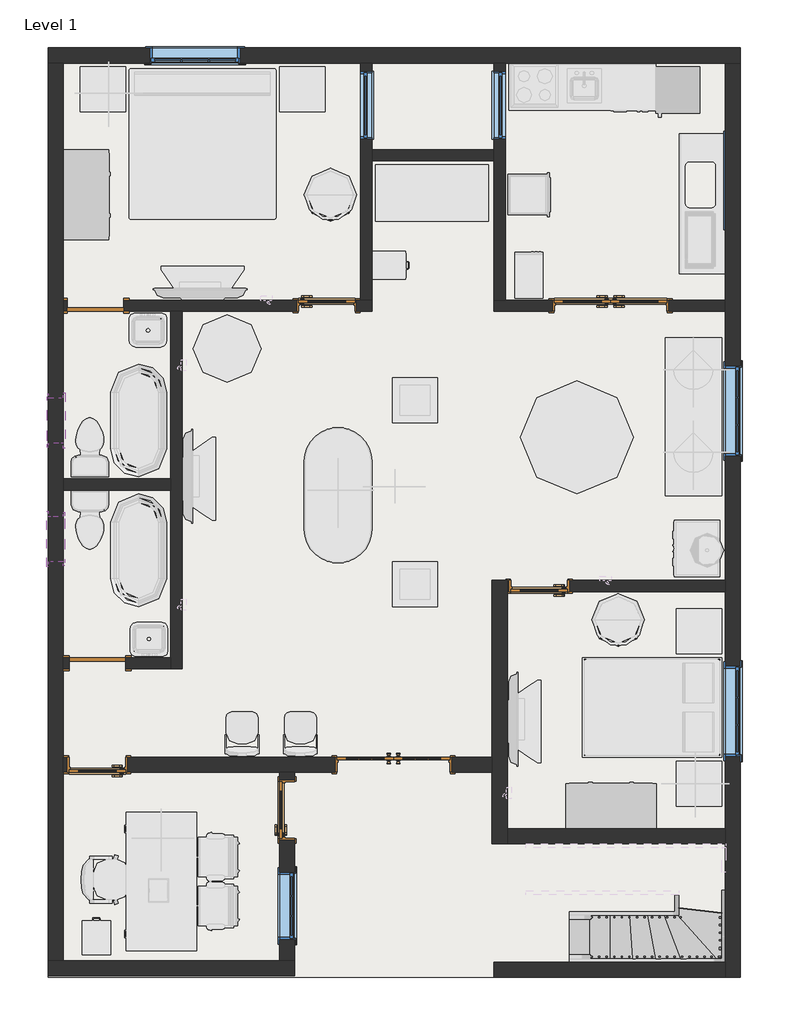
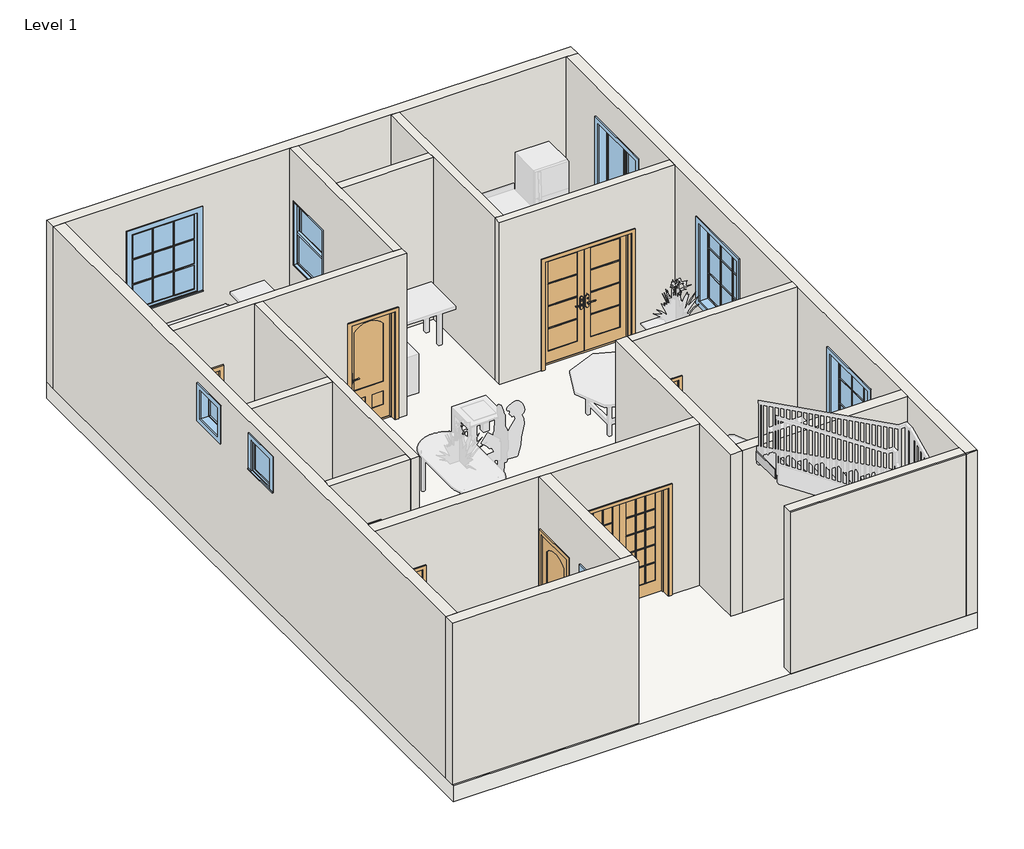
# One storey, part 1 of 3: 18 walls, 9 windows, 8 doors, 1 slab, 1 stair flight.
"""IFC4 building model written with IfcOpenShell, lengths in millimetres."""

from ifc_helpers import new_model, si_unit, frame, origin, origin_with_axes, place, context, project, spatial, polyline, outline, extrude, faceted_brep, transform, mapped, element, save
from components import door_41326d50, door_4b146b56, door_94998e6c, door_9d00318c, door_255cab33, door_059fdd7e, stair_flight_08a12ea7, window_29c06734, window_4f803b43, window_cfa1ffdd, window_0862ab64, window_d6fe7540, window_e41d21a6

model = new_model("IFC4")

# Units and contexts
model_context = context("Model", 3, world=origin())
ifc_project = project(units=[si_unit("LENGTHUNIT", "METRE", prefix="MILLI")], contexts=[model_context])

# Site, building, storey
site = spatial("IfcSite", under=ifc_project)
building = spatial("IfcBuilding", under=site)
storey = spatial("IfcBuildingStorey", under=building, Name="Level 1", Elevation=0.0)

# Doors
placement = place(None, origin())
door_shape = door_41326d50(model_context)
element("IfcDoor", 1, ObjectType="30\" x 80\"", at=placement, inside=storey, context=model_context, shape_type="MappedRepresentation", body=[
    mapped(door_shape, transform((-5998.3041596, 3065.8845092, 0.0), x_axis=(1.0, 0.0, 0.0), y_axis=(0.0, 1.0, 0.0), z_axis=(0.0, 0.0, 1.0))),
])
element("IfcDoor", 2, ObjectType="30\" x 80\"", at=placement, inside=storey, context=model_context, shape_type="MappedRepresentation", body=[
    mapped(door_shape, transform((-3436.0791596, 2459.4595092, 0.0), x_axis=(0.0, -1.0, 0.0), y_axis=(1.0, 0.0, 0.0), z_axis=(0.0, 0.0, 1.0))),
])
door_2_shape = door_4b146b56(model_context)
element("IfcDoor", 3, ObjectType="30\" x 80\"", at=placement, inside=storey, context=model_context, shape_type="MappedRepresentation", body=[
    mapped(door_2_shape, transform((-29.3041596, 5478.8845092, 0.0), x_axis=(1.0, 0.0, 0.0), y_axis=(0.0, 1.0, 0.0), z_axis=(0.0, 0.0, 1.0))),
])
element("IfcDoor", 4, ObjectType="30\" x 80\"", at=placement, inside=storey, context=model_context, shape_type="MappedRepresentation", body=[
    mapped(door_2_shape, transform((-2899.5041596, 9269.8345092, 0.0), x_axis=(-1.0, 0.0, 0.0), y_axis=(0.0, -1.0, 0.0), z_axis=(0.0, 0.0, 1.0))),
])
door_3_shape = door_94998e6c(model_context)
element("IfcDoor", 5, ObjectType="Door-Exterior-Double-Full Glass-Wood_Clad : 60\" x 80\"", at=placement, inside=storey, context=model_context, shape_type="MappedRepresentation", body=[
    mapped(door_3_shape, transform((935.8958404, 9269.8345092, 0.0), x_axis=(1.0, 0.0, 0.0), y_axis=(0.0, 1.0, 0.0), z_axis=(0.0, 0.0, 1.0))),
])
door_4_shape = door_9d00318c(model_context)
element("IfcDoor", 6, ObjectType="Door-Interior-Double-Full Glass-Wood : 60\" x 80\"", at=placement, inside=storey, context=model_context, shape_type="MappedRepresentation", body=[
    mapped(door_4_shape, transform((-1997.8041596, 3072.2345092, 0.0), x_axis=(1.0, 0.0, 0.0), y_axis=(0.0, 1.0, 0.0), z_axis=(0.0, 0.0, 1.0))),
])
door_5_shape = door_255cab33(model_context)
element("IfcDoor", 7, ObjectType="Single-Flush : 30\" x 80\"", at=placement, inside=storey, context=model_context, shape_type="MappedRepresentation", body=[
    mapped(door_5_shape, transform((-5998.3041596, 4440.6595092, 0.0), x_axis=(-1.0, 0.0, 0.0), y_axis=(0.0, -1.0, 0.0), z_axis=(0.0, 0.0, 1.0))),
])
door_6_shape = door_059fdd7e(model_context)
element("IfcDoor", 8, ObjectType="Single-Flush : 30\" x 80\"", at=placement, inside=storey, context=model_context, shape_type="MappedRepresentation", body=[
    mapped(door_6_shape, transform((-6023.7041596, 9266.6595092, 0.0), x_axis=(-1.0, 0.0, 0.0), y_axis=(0.0, -1.0, 0.0), z_axis=(0.0, 0.0, 1.0))),
])

# Slab
element("IfcSlab", 9, ObjectType="Generic - 12\"", at=placement, inside=storey, context=model_context, shape_type="SweptSolid", body=[
    extrude(outline(polyline([(2688.4958404, 12746.4595092), (2688.4958404, 198.8595092), (-6658.7041596, 198.8595092), (-6658.7041596, 12746.4595092), (2688.4958404, 12746.4595092)])), frame((0.0, 0.0, -304.8), z_axis=(0.0, 0.0, 1.0), x_axis=(1.0, 0.0, 0.0)), (0.0, 0.0, 1.0), 304.8),
])

# Stair flight
stair_flight_shape = stair_flight_08a12ea7(model_context)
element("IfcStairFlight", 10, ObjectType="2\" Tread 1\" Nosing 1/4\" Riser", at=placement, inside=storey, context=model_context, shape_type="MappedRepresentation", body=[
    mapped(stair_flight_shape, transform((0.0, 0.0, 0.0), x_axis=(1.0, 0.0, 0.0), y_axis=(0.0, 1.0, 0.0), z_axis=(0.0, 0.0, 1.0))),
])

# Walls
element("IfcWall", 11, ObjectType="Generic - 8\"", at=placement, inside=storey, context=model_context, shape_type="Brep", body=[
    faceted_brep([(-6658.7041596, 12543.2595092, 0.0), (-6455.5041596, 12543.2595092, 0.0), (-2442.3041596, 12543.2595092, 0.0), (-2289.9041596, 12543.2595092, 0.0), (-638.9041596, 12543.2595092, 0.0), (-486.5041596, 12543.2595092, 0.0), (2485.2958404, 12543.2595092, 0.0), (2688.4958404, 12543.2595092, 0.0), (2688.4958404, 12543.2595092, 3048.0), (2485.2958404, 12543.2595092, 3048.0), (-486.5041596, 12543.2595092, 3048.0), (-638.9041596, 12543.2595092, 3048.0), (-2289.9041596, 12543.2595092, 3048.0), (-2442.3041596, 12543.2595092, 3048.0), (-6455.5041596, 12543.2595092, 3048.0), (-6658.7041596, 12543.2595092, 3048.0), (-4067.9041596, 12543.2595092, 2438.4), (-4067.9041596, 12543.2595092, 914.4), (-5287.1041596, 12543.2595092, 914.4), (-5287.1041596, 12543.2595092, 2438.4), (-6658.7041596, 12746.4595092, 0.0), (-6658.7041596, 12746.4595092, 3048.0), (2688.4958404, 12746.4595092, 3048.0), (2688.4958404, 12746.4595092, 0.0), (-4067.9041596, 12746.4595092, 2438.4), (-5287.1041596, 12746.4595092, 2438.4), (-5287.1041596, 12746.4595092, 914.4), (-4067.9041596, 12746.4595092, 914.4)], [[[0, 1, 2, 3, 4, 5, 6, 7, 8, 9, 10, 11, 12, 13, 14, 15], [16, 17, 18, 19]], [[20, 21, 22, 23], [24, 25, 26, 27]], [[7, 6, 5, 4, 3, 2, 1, 0, 20, 23]], [[8, 7, 23, 22]], [[0, 15, 21, 20]], [[15, 14, 13, 12, 11, 10, 9, 8, 22, 21]], [[17, 16, 24, 27]], [[18, 17, 27, 26]], [[19, 18, 26, 25]], [[16, 19, 25, 24]]]),
])
element("IfcWall", 12, ObjectType="Generic - 8\"", at=placement, inside=storey, context=model_context, shape_type="Brep", body=[
    faceted_brep([(2485.2958404, 12543.2595092, 0.0), (2485.2958404, 9342.8595092, 0.0), (2485.2958404, 9190.4595092, 0.0), (2485.2958404, 5558.2595092, 0.0), (2485.2958404, 5405.8595092, 0.0), (2485.2958404, 2205.4595092, 0.0), (2485.2958404, 2002.2595092, 0.0), (2485.2958404, 402.0595092, 0.0), (2485.2958404, 198.8595092, 0.0), (2485.2958404, 198.8595092, 3048.0), (2485.2958404, 224.2595092, 3048.0), (2485.2958404, 402.0595092, 3048.0), (2485.2958404, 2002.2595092, 3048.0), (2485.2958404, 2205.4595092, 3048.0), (2485.2958404, 5405.8595092, 3048.0), (2485.2958404, 5558.2595092, 3048.0), (2485.2958404, 9190.4595092, 3048.0), (2485.2958404, 9342.8595092, 3048.0), (2485.2958404, 12543.2595092, 3048.0), (2485.2958404, 3183.3595092, 2438.4), (2485.2958404, 3183.3595092, 914.4), (2485.2958404, 4402.5595092, 914.4), (2485.2958404, 4402.5595092, 2438.4), (2485.2958404, 7234.6595092, 2438.4), (2485.2958404, 7234.6595092, 914.4), (2485.2958404, 8453.8595092, 914.4), (2485.2958404, 8453.8595092, 2438.4), (2485.2958404, 10346.1595092, 2438.4), (2485.2958404, 10346.1595092, 1219.2), (2485.2958404, 11565.3595092, 1219.2), (2485.2958404, 11565.3595092, 2438.4), (2688.4958404, 12543.2595092, 0.0), (2688.4958404, 12543.2595092, 3048.0), (2688.4958404, 224.2595092, 3048.0), (2688.4958404, 198.8595092, 3048.0), (2688.4958404, 198.8595092, 0.0), (2688.4958404, 3183.3595092, 2438.4), (2688.4958404, 4402.5595092, 2438.4), (2688.4958404, 4402.5595092, 914.4), (2688.4958404, 3183.3595092, 914.4), (2688.4958404, 7234.6595092, 2438.4), (2688.4958404, 8453.8595092, 2438.4), (2688.4958404, 8453.8595092, 914.4), (2688.4958404, 7234.6595092, 914.4), (2688.4958404, 10346.1595092, 2438.4), (2688.4958404, 11565.3595092, 2438.4), (2688.4958404, 11565.3595092, 1219.2), (2688.4958404, 10346.1595092, 1219.2)], [[[0, 1, 2, 3, 4, 5, 6, 7, 8, 9, 10, 11, 12, 13, 14, 15, 16, 17, 18], [19, 20, 21, 22], [23, 24, 25, 26], [27, 28, 29, 30]], [[31, 32, 33, 34, 35], [36, 37, 38, 39], [40, 41, 42, 43], [44, 45, 46, 47]], [[8, 7, 6, 5, 4, 3, 2, 1, 0, 31, 35]], [[0, 18, 32, 31]], [[9, 8, 35, 34]], [[10, 9, 34, 33]], [[18, 17, 16, 15, 14, 13, 12, 11, 10, 33, 32]], [[20, 19, 36, 39]], [[21, 20, 39, 38]], [[22, 21, 38, 37]], [[19, 22, 37, 36]], [[24, 23, 40, 43]], [[25, 24, 43, 42]], [[26, 25, 42, 41]], [[23, 26, 41, 40]], [[28, 27, 44, 47]], [[29, 28, 47, 46]], [[30, 29, 46, 45]], [[27, 30, 45, 44]]]),
])
element("IfcWall", 13, ObjectType="Generic - 8\"", at=placement, inside=storey, context=model_context, shape_type="SweptSolid", body=[
    extrude(outline(polyline([(402.0595092, 3048.0), (402.0595092, 0.0), (198.8595092, 0.0), (198.8595092, 3048.0), (224.2595092, 3048.0), (402.0595092, 3048.0)])), frame((-638.9041596, 0.0, 0.0), z_axis=(1.0, 0.0, 0.0), x_axis=(0.0, 1.0, 0.0)), (0.0, 0.0, 1.0), 3124.2),
])
element("IfcWall", 14, ObjectType="Generic - 8\"", at=placement, inside=storey, context=model_context, shape_type="Brep", body=[
    faceted_brep([(-6455.5041596, 427.4595092, 0.0), (-6455.5041596, 2967.4595092, 0.0), (-6455.5041596, 3170.6595092, 0.0), (-6455.5041596, 4364.4595092, 0.0), (-6455.5041596, 4516.8595092, 0.0), (-6455.5041596, 6777.4595092, 0.0), (-6455.5041596, 6929.8595092, 0.0), (-6455.5041596, 9190.4595092, 0.0), (-6455.5041596, 9342.8595092, 0.0), (-6455.5041596, 12543.2595092, 0.0), (-6455.5041596, 12543.2595092, 3048.0), (-6455.5041596, 9342.8595092, 3048.0), (-6455.5041596, 9190.4595092, 3048.0), (-6455.5041596, 6929.8595092, 3048.0), (-6455.5041596, 6777.4595092, 3048.0), (-6455.5041596, 4516.8595092, 3048.0), (-6455.5041596, 4364.4595092, 3048.0), (-6455.5041596, 3170.6595092, 3048.0), (-6455.5041596, 2967.4595092, 3048.0), (-6455.5041596, 427.4595092, 3048.0), (-6455.5041596, 6421.8595092, 2768.6), (-6455.5041596, 6421.8595092, 2159.0), (-6455.5041596, 5812.2595092, 2159.0), (-6455.5041596, 5812.2595092, 2768.6), (-6455.5041596, 7412.4595092, 2768.6), (-6455.5041596, 8022.0595092, 2768.6), (-6455.5041596, 8022.0595092, 2159.0), (-6455.5041596, 7412.4595092, 2159.0), (-6658.7041596, 427.4595092, 0.0), (-6658.7041596, 427.4595092, 3048.0), (-6658.7041596, 12543.2595092, 3048.0), (-6658.7041596, 12543.2595092, 0.0), (-6658.7041596, 6421.8595092, 2768.6), (-6658.7041596, 5812.2595092, 2768.6), (-6658.7041596, 5812.2595092, 2159.0), (-6658.7041596, 6421.8595092, 2159.0), (-6658.7041596, 7412.4595092, 2768.6), (-6658.7041596, 7412.4595092, 2159.0), (-6658.7041596, 8022.0595092, 2159.0), (-6658.7041596, 8022.0595092, 2768.6)], [[[0, 1, 2, 3, 4, 5, 6, 7, 8, 9, 10, 11, 12, 13, 14, 15, 16, 17, 18, 19], [20, 21, 22, 23], [24, 25, 26, 27]], [[28, 29, 30, 31], [32, 33, 34, 35], [36, 37, 38, 39]], [[9, 8, 7, 6, 5, 4, 3, 2, 1, 0, 28, 31]], [[10, 9, 31, 30]], [[0, 19, 29, 28]], [[19, 18, 17, 16, 15, 14, 13, 12, 11, 10, 30, 29]], [[21, 20, 32, 35]], [[22, 21, 35, 34]], [[23, 22, 34, 33]], [[20, 23, 33, 32]], [[37, 36, 24, 27]], [[38, 37, 27, 26]], [[39, 38, 26, 25]], [[36, 39, 25, 24]]]),
])
element("IfcWall", 15, ObjectType="Generic - 8\"", at=placement, inside=storey, context=model_context, shape_type="Brep", body=[
    faceted_brep([(-6455.5041596, 2967.4595092, 3048.0), (-6455.5041596, 2967.4595092, 0.0), (-6404.7041596, 2967.4595092, 0.0), (-6404.7041596, 2967.4595092, 2057.4), (-5591.9041596, 2967.4595092, 2057.4), (-5591.9041596, 2967.4595092, 0.0), (-3534.5041596, 2967.4595092, 0.0), (-3331.3041596, 2967.4595092, 0.0), (-2785.2041596, 2967.4595092, 0.0), (-2785.2041596, 2967.4595092, 2057.4), (-1210.4041596, 2967.4595092, 2057.4), (-1210.4041596, 2967.4595092, 0.0), (-664.3041596, 2967.4595092, 0.0), (-664.3041596, 2967.4595092, 3048.0), (-3331.3041596, 2967.4595092, 3048.0), (-3534.5041596, 2967.4595092, 3048.0), (-6455.5041596, 3170.6595092, 0.0), (-6455.5041596, 3170.6595092, 3048.0), (-664.3041596, 3170.6595092, 3048.0), (-664.3041596, 3170.6595092, 0.0), (-1210.4041596, 3170.6595092, 0.0), (-1210.4041596, 3170.6595092, 2057.4), (-2785.2041596, 3170.6595092, 2057.4), (-2785.2041596, 3170.6595092, 0.0), (-5591.9041596, 3170.6595092, 0.0), (-5591.9041596, 3170.6595092, 2057.4), (-6404.7041596, 3170.6595092, 2057.4), (-6404.7041596, 3170.6595092, 0.0)], [[[0, 1, 2, 3, 4, 5, 6, 7, 8, 9, 10, 11, 12, 13, 14, 15]], [[16, 17, 18, 19, 20, 21, 22, 23, 24, 25, 26, 27]], [[1, 16, 27, 2]], [[19, 12, 11, 20]], [[23, 8, 7, 6, 5, 24]], [[1, 0, 17, 16]], [[13, 12, 19, 18]], [[10, 21, 20, 11]], [[21, 10, 9, 22]], [[22, 9, 8, 23]], [[4, 25, 24, 5]], [[25, 4, 3, 26]], [[26, 3, 2, 27]], [[0, 15, 14, 13, 18, 17]]]),
])
element("IfcWall", 16, ObjectType="Generic - 8\"", at=placement, inside=storey, context=model_context, shape_type="SweptSolid", body=[
    extrude(outline(polyline([(2485.2958404, 2002.2595092), (-461.1041596, 2002.2595092), (-461.1041596, 2205.4595092), (2485.2958404, 2205.4595092), (2485.2958404, 2002.2595092)])), origin_with_axes(), (0.0, 0.0, 1.0), 3048.0),
])
element("IfcWall", 17, ObjectType="Generic - 8\"", at=placement, inside=storey, context=model_context, shape_type="Brep", body=[
    faceted_brep([(-664.3041596, 5558.2595092, 0.0), (-664.3041596, 3170.6595092, 0.0), (-664.3041596, 2967.4595092, 0.0), (-664.3041596, 2002.2595092, 0.0), (-664.3041596, 2002.2595092, 3048.0), (-664.3041596, 2967.4595092, 3048.0), (-664.3041596, 3170.6595092, 3048.0), (-664.3041596, 5558.2595092, 3048.0), (-461.1041596, 5558.2595092, 0.0), (-461.1041596, 5558.2595092, 3048.0), (-461.1041596, 5405.8595092, 3048.0), (-461.1041596, 2205.4595092, 3048.0), (-461.1041596, 2002.2595092, 3048.0), (-461.1041596, 2002.2595092, 0.0), (-461.1041596, 2205.4595092, 0.0), (-461.1041596, 5405.8595092, 0.0)], [[[0, 1, 2, 3, 4, 5, 6, 7]], [[8, 9, 10, 11, 12, 13, 14, 15]], [[3, 2, 1, 0, 8, 15, 14, 13]], [[4, 3, 13, 12]], [[0, 7, 9, 8]], [[7, 6, 5, 4, 12, 11, 10, 9]]]),
])
element("IfcWall", 18, ObjectType="Generic - 8\"", at=placement, inside=storey, context=model_context, shape_type="Brep", body=[
    faceted_brep([(-3331.3041596, 427.4595092, 0.0), (-3534.5041596, 427.4595092, 0.0), (-6455.5041596, 427.4595092, 0.0), (-6658.7041596, 427.4595092, 0.0), (-6658.7041596, 427.4595092, 3048.0), (-6455.5041596, 427.4595092, 3048.0), (-3534.5041596, 427.4595092, 3048.0), (-3331.3041596, 427.4595092, 3048.0), (-3331.3041596, 224.2595092, 0.0), (-3331.3041596, 224.2595092, 3048.0), (-6658.7041596, 224.2595092, 3048.0), (-6658.7041596, 224.2595092, 0.0)], [[[0, 1, 2, 3, 4, 5, 6, 7]], [[8, 9, 10, 11]], [[3, 2, 1, 0, 8, 11]], [[4, 3, 11, 10]], [[7, 6, 5, 4, 10, 9]], [[0, 7, 9, 8]]]),
])
element("IfcWall", 19, ObjectType="Generic - 8\"", at=placement, inside=storey, context=model_context, shape_type="SweptSolid", body=[
    extrude(outline(polyline([(427.4595092, 0.0), (427.4595092, 3048.0), (2967.4595092, 3048.0), (2967.4595092, 0.0), (2865.8595092, 0.0), (2865.8595092, 2057.4), (2053.0595092, 2057.4), (2053.0595092, 0.0), (427.4595092, 0.0)]), holes=[polyline([(706.8595092, 2133.6), (706.8595092, 914.4), (1621.2595092, 914.4), (1621.2595092, 2133.6), (706.8595092, 2133.6)])]), frame((-3534.5041596, 0.0, 0.0), z_axis=(1.0, 0.0, 0.0), x_axis=(0.0, 1.0, 0.0)), (0.0, 0.0, 1.0), 203.2),
])
element("IfcWall", 20, ObjectType="INNER WALL", at=placement, inside=storey, context=model_context, shape_type="Brep", body=[
    faceted_brep([(-638.9041596, 9342.8595092, 0.0), (-638.9041596, 9342.8595092, 3048.0), (-486.5041596, 9342.8595092, 3048.0), (2485.2958404, 9342.8595092, 3048.0), (2485.2958404, 9342.8595092, 0.0), (1723.2958404, 9342.8595092, 0.0), (1723.2958404, 9342.8595092, 2057.4), (148.4958404, 9342.8595092, 2057.4), (148.4958404, 9342.8595092, 0.0), (-486.5041596, 9342.8595092, 0.0), (-638.9041596, 9190.4595092, 3048.0), (-638.9041596, 9190.4595092, 0.0), (148.4958404, 9190.4595092, 0.0), (148.4958404, 9190.4595092, 2057.4), (1723.2958404, 9190.4595092, 2057.4), (1723.2958404, 9190.4595092, 0.0), (2485.2958404, 9190.4595092, 0.0), (2485.2958404, 9190.4595092, 3048.0)], [[[0, 1, 2, 3, 4, 5, 6, 7, 8, 9]], [[10, 11, 12, 13, 14, 15, 16, 17]], [[11, 0, 9, 8, 12]], [[4, 16, 15, 5]], [[1, 0, 11, 10]], [[4, 3, 17, 16]], [[14, 6, 5, 15]], [[6, 14, 13, 7]], [[7, 13, 12, 8]], [[3, 2, 1, 10, 17]]]),
])
element("IfcWall", 21, ObjectType="INNER WALL", at=placement, inside=storey, context=model_context, shape_type="Brep", body=[
    faceted_brep([(-486.5041596, 9342.8595092, 0.0), (-486.5041596, 12543.2595092, 0.0), (-486.5041596, 12543.2595092, 3048.0), (-486.5041596, 9342.8595092, 3048.0), (-486.5041596, 12428.9595092, 2133.6), (-486.5041596, 12428.9595092, 914.4), (-486.5041596, 11514.5595092, 914.4), (-486.5041596, 11514.5595092, 2133.6), (-638.9041596, 9342.8595092, 0.0), (-638.9041596, 9342.8595092, 3048.0), (-638.9041596, 11222.4595092, 3048.0), (-638.9041596, 11374.8595092, 3048.0), (-638.9041596, 12543.2595092, 3048.0), (-638.9041596, 12543.2595092, 0.0), (-638.9041596, 11374.8595092, 0.0), (-638.9041596, 11222.4595092, 0.0), (-638.9041596, 12428.9595092, 2133.6), (-638.9041596, 11514.5595092, 2133.6), (-638.9041596, 11514.5595092, 914.4), (-638.9041596, 12428.9595092, 914.4)], [[[0, 1, 2, 3], [4, 5, 6, 7]], [[8, 9, 10, 11, 12, 13, 14, 15], [16, 17, 18, 19]], [[1, 0, 8, 15, 14, 13]], [[2, 1, 13, 12]], [[0, 3, 9, 8]], [[3, 2, 12, 11, 10, 9]], [[5, 4, 16, 19]], [[6, 5, 19, 18]], [[7, 6, 18, 17]], [[4, 7, 17, 16]]]),
])
element("IfcWall", 22, ObjectType="INNER WALL", at=placement, inside=storey, context=model_context, shape_type="Brep", body=[
    faceted_brep([(-2289.9041596, 9342.8595092, 0.0), (-2289.9041596, 11222.4595092, 0.0), (-2289.9041596, 11374.8595092, 0.0), (-2289.9041596, 12543.2595092, 0.0), (-2289.9041596, 12543.2595092, 3048.0), (-2289.9041596, 11374.8595092, 3048.0), (-2289.9041596, 11222.4595092, 3048.0), (-2289.9041596, 9342.8595092, 3048.0), (-2289.9041596, 11514.5595092, 2133.6), (-2289.9041596, 12428.9595092, 2133.6), (-2289.9041596, 12428.9595092, 914.4), (-2289.9041596, 11514.5595092, 914.4), (-2442.3041596, 9342.8595092, 0.0), (-2442.3041596, 9342.8595092, 3048.0), (-2442.3041596, 12543.2595092, 3048.0), (-2442.3041596, 12543.2595092, 0.0), (-2442.3041596, 11514.5595092, 2133.6), (-2442.3041596, 11514.5595092, 914.4), (-2442.3041596, 12428.9595092, 914.4), (-2442.3041596, 12428.9595092, 2133.6)], [[[0, 1, 2, 3, 4, 5, 6, 7], [8, 9, 10, 11]], [[12, 13, 14, 15], [16, 17, 18, 19]], [[3, 2, 1, 0, 12, 15]], [[0, 7, 13, 12]], [[4, 3, 15, 14]], [[7, 6, 5, 4, 14, 13]], [[17, 16, 8, 11]], [[18, 17, 11, 10]], [[19, 18, 10, 9]], [[16, 19, 9, 8]]]),
])
element("IfcWall", 23, ObjectType="INNER WALL", at=placement, inside=storey, context=model_context, shape_type="Brep", body=[
    faceted_brep([(-5007.7041596, 9190.4595092, 0.0), (-5007.7041596, 6929.8595092, 0.0), (-5007.7041596, 6777.4595092, 0.0), (-5007.7041596, 4516.8595092, 0.0), (-5007.7041596, 4364.4595092, 0.0), (-5007.7041596, 4364.4595092, 3048.0), (-5007.7041596, 4516.8595092, 3048.0), (-5007.7041596, 6777.4595092, 3048.0), (-5007.7041596, 6929.8595092, 3048.0), (-5007.7041596, 9190.4595092, 3048.0), (-4855.3041596, 9190.4595092, 0.0), (-4855.3041596, 9190.4595092, 3048.0), (-4855.3041596, 4364.4595092, 3048.0), (-4855.3041596, 4364.4595092, 0.0)], [[[0, 1, 2, 3, 4, 5, 6, 7, 8, 9]], [[10, 11, 12, 13]], [[4, 3, 2, 1, 0, 10, 13]], [[0, 9, 11, 10]], [[5, 4, 13, 12]], [[9, 8, 7, 6, 5, 12, 11]]]),
])
element("IfcWall", 24, ObjectType="INNER WALL", at=placement, inside=storey, context=model_context, shape_type="SweptSolid", body=[
    extrude(outline(polyline([(0.0, -5007.7041596), (3048.0, -5007.7041596), (3048.0, -6455.5041596), (0.0, -6455.5041596), (0.0, -6379.3041596), (2032.0, -6379.3041596), (2032.0, -5617.3041596), (0.0, -5617.3041596), (0.0, -5007.7041596)])), frame((0.0, 4364.4595092, 0.0), z_axis=(0.0, 1.0, 0.0), x_axis=(0.0, 0.0, 1.0)), (0.0, 0.0, 1.0), 152.4),
])
element("IfcWall", 25, ObjectType="INNER WALL", at=placement, inside=storey, context=model_context, shape_type="SweptSolid", body=[
    extrude(outline(polyline([(-6455.5041596, 6929.8595092), (-5007.7041596, 6929.8595092), (-5007.7041596, 6777.4595092), (-6455.5041596, 6777.4595092), (-6455.5041596, 6929.8595092)])), origin_with_axes(), (0.0, 0.0, 1.0), 3048.0),
])
element("IfcWall", 26, ObjectType="INNER WALL", at=placement, inside=storey, context=model_context, shape_type="SweptSolid", body=[
    extrude(outline(polyline([(0.0, 2485.2958404), (3048.0, 2485.2958404), (3048.0, -461.1041596), (0.0, -461.1041596), (0.0, -435.7041596), (2057.4, -435.7041596), (2057.4, 377.0958404), (0.0, 377.0958404), (0.0, 2485.2958404)])), frame((0.0, 5405.8595092, 0.0), z_axis=(0.0, 1.0, 0.0), x_axis=(0.0, 0.0, 1.0)), (0.0, 0.0, 1.0), 152.4),
])
element("IfcWall", 27, ObjectType="INNER WALL", at=placement, inside=storey, context=model_context, shape_type="SweptSolid", body=[
    extrude(outline(polyline([(-2289.9041596, 11374.8595092), (-638.9041596, 11374.8595092), (-638.9041596, 11222.4595092), (-2289.9041596, 11222.4595092), (-2289.9041596, 11374.8595092)])), origin_with_axes(), (0.0, 0.0, 1.0), 3048.0),
])
element("IfcWall", 28, ObjectType="INNER WALL", at=placement, inside=storey, context=model_context, shape_type="Brep", body=[
    faceted_brep([(-2289.9041596, 9342.8595092, 3048.0), (-2289.9041596, 9342.8595092, 0.0), (-2442.3041596, 9342.8595092, 0.0), (-2493.1041596, 9342.8595092, 0.0), (-2493.1041596, 9342.8595092, 2057.4), (-3305.9041596, 9342.8595092, 2057.4), (-3305.9041596, 9342.8595092, 0.0), (-5642.7041596, 9342.8595092, 0.0), (-5642.7041596, 9342.8595092, 2032.0), (-6404.7041596, 9342.8595092, 2032.0), (-6404.7041596, 9342.8595092, 0.0), (-6455.5041596, 9342.8595092, 0.0), (-6455.5041596, 9342.8595092, 3048.0), (-2442.3041596, 9342.8595092, 3048.0), (-2289.9041596, 9190.4595092, 0.0), (-2289.9041596, 9190.4595092, 3048.0), (-4855.3041596, 9190.4595092, 3048.0), (-5007.7041596, 9190.4595092, 3048.0), (-6455.5041596, 9190.4595092, 3048.0), (-6455.5041596, 9190.4595092, 0.0), (-6404.7041596, 9190.4595092, 0.0), (-6404.7041596, 9190.4595092, 2032.0), (-5642.7041596, 9190.4595092, 2032.0), (-5642.7041596, 9190.4595092, 0.0), (-5007.7041596, 9190.4595092, 0.0), (-4855.3041596, 9190.4595092, 0.0), (-3305.9041596, 9190.4595092, 0.0), (-3305.9041596, 9190.4595092, 2057.4), (-2493.1041596, 9190.4595092, 2057.4), (-2493.1041596, 9190.4595092, 0.0)], [[[0, 1, 2, 3, 4, 5, 6, 7, 8, 9, 10, 11, 12, 13]], [[14, 15, 16, 17, 18, 19, 20, 21, 22, 23, 24, 25, 26, 27, 28, 29]], [[1, 14, 29, 3, 2]], [[19, 11, 10, 20]], [[23, 7, 6, 26, 25, 24]], [[1, 0, 15, 14]], [[12, 11, 19, 18]], [[23, 22, 8, 7]], [[22, 21, 9, 8]], [[21, 20, 10, 9]], [[5, 27, 26, 6]], [[27, 5, 4, 28]], [[28, 4, 3, 29]], [[0, 13, 12, 18, 17, 16, 15]]]),
])

# Windows
window_shape = window_29c06734(model_context)
element("IfcWindow", 29, ObjectType="Casement 3x3 with Trim : 36\" x 48\"", at=placement, inside=storey, context=model_context, shape_type="MappedRepresentation", body=[
    mapped(window_shape, transform((-3432.9041596, 1164.0595092, 0.0), x_axis=(0.0, -1.0, 0.0), y_axis=(1.0, 0.0, 0.0), z_axis=(0.0, 0.0, 1.0))),
])
window_2_shape = window_4f803b43(model_context)
element("IfcWindow", 30, ObjectType="Casement 3x3 with Trim : 48\" x 60\"", at=placement, inside=storey, context=model_context, shape_type="MappedRepresentation", body=[
    mapped(window_2_shape, transform((-4677.5041596, 12644.8595092, 304.8), x_axis=(1.0, 0.0, 0.0), y_axis=(0.0, 1.0, 0.0), z_axis=(0.0, 0.0, 1.0))),
])
window_3_shape = window_cfa1ffdd(model_context)
element("IfcWindow", 31, ObjectType="Casement 3x3 with Trim : 48\" x 60\"", at=placement, inside=storey, context=model_context, shape_type="MappedRepresentation", body=[
    mapped(window_3_shape, transform((2586.8958404, 3792.9595092, 304.8), x_axis=(0.0, -1.0, 0.0), y_axis=(1.0, 0.0, 0.0), z_axis=(0.0, 0.0, 1.0))),
])
element("IfcWindow", 32, ObjectType="Casement 3x3 with Trim : 48\" x 60\"", at=placement, inside=storey, context=model_context, shape_type="MappedRepresentation", body=[
    mapped(window_3_shape, transform((2586.8958404, 7844.2595092, 304.8), x_axis=(0.0, -1.0, 0.0), y_axis=(1.0, 0.0, 0.0), z_axis=(0.0, 0.0, 1.0))),
])
window_4_shape = window_0862ab64(model_context)
element("IfcWindow", 33, ObjectType="Casement Dbl with Trim : 48\" x 48\"", at=placement, inside=storey, context=model_context, shape_type="MappedRepresentation", body=[
    mapped(window_4_shape, transform((2567.8458404, 10955.7595092, 304.8), x_axis=(0.0, -1.0, 0.0), y_axis=(1.0, 0.0, 0.0), z_axis=(0.0, 0.0, 1.0))),
])
window_5_shape = window_d6fe7540(model_context)
element("IfcWindow", 34, ObjectType="Double Hung : 36\" x 48\"", at=placement, inside=storey, context=model_context, shape_type="MappedRepresentation", body=[
    mapped(window_5_shape, transform((-562.7041596, 11971.7595092, 0.0), x_axis=(0.0, 1.0, 0.0), y_axis=(-1.0, 0.0, 0.0), z_axis=(0.0, 0.0, 1.0))),
])
element("IfcWindow", 35, ObjectType="Double Hung : 36\" x 48\"", at=placement, inside=storey, context=model_context, shape_type="MappedRepresentation", body=[
    mapped(window_5_shape, transform((-2366.1041596, 11971.7595092, 0.0), x_axis=(0.0, -1.0, 0.0), y_axis=(1.0, 0.0, 0.0), z_axis=(0.0, 0.0, 1.0))),
])
window_6_shape = window_e41d21a6(model_context)
element("IfcWindow", 36, ObjectType="Transom with Trim : 24\" x 24\"", at=placement, inside=storey, context=model_context, shape_type="MappedRepresentation", body=[
    mapped(window_6_shape, transform((-6557.1041596, 6155.1595092, 0.0), x_axis=(0.0, 1.0, 0.0), y_axis=(-1.0, 0.0, 0.0), z_axis=(0.0, 0.0, 1.0))),
])
element("IfcWindow", 37, ObjectType="Transom with Trim : 24\" x 24\"", at=placement, inside=storey, context=model_context, shape_type="MappedRepresentation", body=[
    mapped(window_6_shape, transform((-6557.1041596, 7679.1595092, 0.0), x_axis=(0.0, -1.0, 0.0), y_axis=(1.0, 0.0, 0.0), z_axis=(0.0, 0.0, 1.0))),
])

save(model, "model.ifc")

# Revit data of these elements
# Type "30\" x 80\""
#   Type Mark = "9"
#   Assembly Code = "B2030100"
#   Analytic Construction = "French door, wood frame with single glass"
#   Threshold Offset [instance default] = 0' - 0 1/2"
#   Thickness = 0' - 1 3/8"
#   Thermal Resistance (R) = 1.0696 (h·ft²·°F)/BTU
#   Swing Angle [instance default] = 90.00°
#   Stiles = 0' - 4 3/4"
#   Rough Width = 2' - 8"
#   Rough Height = 6' - 9"
#   Radius = 1' - 1.00625"
#   Lock Rail = 0' - 7 1/8"
#   Height = 6' - 8"
#   Width = 2' - 6"
#   Heat Transfer Coefficient (U) = 0.9350 BTU/(h·ft²·°F)
#   Door Offset [instance default] = 0' - 0"
#   Bottom Rail = 0' - 9 1/2"
#   Threshold [instance default] = yes
#   Function = 1
#   Exterior Trim [instance default] = yes
#   Trim Material = Cherry
#   Threshold Material = Cherry
#   Panel Material = Cherry
#   Glazing = Glass
#   Frame Material = Cherry
#   Door Handle Material = Aluminum
#   Visual Light Transmittance = 0
#   Solar Heat Gain Coefficient = 0
#   Wall Closure = (empty or 0)
#   Construction Type = (empty or 0)
# Type "Door-Exterior-Double-Full Glass-Wood_Clad : 60\" x 80\""
#   Type Mark = "12"
#   Assembly Code = "B2030100"
#   Analytic Construction = "French door, wood frame with double glass"
#   Top Rail = 0' - 4 11/16"
#   Threshold Offset [instance default] = 0' - 0 1/2"
#   Thickness = 0' - 1 3/8"
#   Thermal Resistance (R) = 1.9158 (h·ft²·°F)/BTU
#   Swing Angle [instance default] = 90.00°
#   Stiles = 0' - 4 3/4"
#   Rough Width = 5' - 2"
#   Rough Height = 6' - 9"
#   Panel Width = 2' - 6"
#   Door Offset [instance default] = 0' - 0"
#   Height = 6' - 8"
#   Width = 5' - 0"
#   Heat Transfer Coefficient (U) = 0.5220 BTU/(h·ft²·°F)
#   Bottom Rail = 0' - 9 1/8"
#   Exterior Trim [instance default] = yes
#   Threshold [instance default] = yes
#   Show Grill [instance default] = yes
#   Function = 1
#   Trim Material = Cherry
#   Threshold Material = Cherry
#   Panel Material = Cherry
#   Glazing = Glass
#   Frame Material = Cherry
#   Door Handle Material = Aluminum
#   Visual Light Transmittance = 0
#   Solar Heat Gain Coefficient = 0
#   Wall Closure = (empty or 0)
#   Construction Type = (empty or 0)
# Type "Door-Interior-Double-Full Glass-Wood : 60\" x 80\""
#   Type Mark = "8"
#   Assembly Code = "C1020300"
#   Analytic Construction = "French door, wood frame with single glass"
#   Top Rail = 0' - 4 11/16"
#   Thickness = 0' - 1 3/8"
#   Thermal Resistance (R) = 1.0696 (h·ft²·°F)/BTU
#   Swing Angle [instance default] = 90.00°
#   Stiles = 0' - 4 3/4"
#   Rough Width = 5' - 2"
#   Rough Height = 6' - 9"
#   Panel Width = 2' - 6"
#   Height = 6' - 8"
#   Width = 5' - 0"
#   Heat Transfer Coefficient (U) = 0.9350 BTU/(h·ft²·°F)
#   Bottom Rail = 0' - 9 1/8"
#   Show Grill [instance default] = yes
#   Trim Material = Cherry
#   Panel Material = Cherry
#   Frame Material = Cherry
#   Door Handle Material = Aluminum
#   Visual Light Transmittance = 0
#   Solar Heat Gain Coefficient = 0
#   Wall Closure = (empty or 0)
#   Function = (empty or 0)
# Type "Single-Flush : 30\" x 80\""
#   Type Mark = "5"
#   Construction Type Id = "MDOOR"
#   Assembly Code = "C1020"
#   Analytic Construction = "Metal"
#   Thickness = 0' - 2"
#   Heat Transfer Coefficient (U) = 0.651978 BTU/(h·ft²·°F)
#   Height = 6' - 8"
#   Trim Projection Ext = 0' - 1"
#   Trim Projection Int = 0' - 1"
#   Trim Width = 0' - 3"
#   Width = 2' - 6"
#   Define Thermal Properties by = 1
#   Door Material = Door - Panel
#   Frame Material = Door - Frame
#   Visual Light Transmittance = 0
#   Solar Heat Gain Coefficient = 0
#   Function = (empty or 0)
#   Wall Closure = (empty or 0)
# Type "Generic - 12\""
#   Assembly Code = "B1010"
#   Function = 0
#   Layers, outside or top first: 1' - 0" no material (function 1)
# Type "Generic - 8\""
#   Assembly Code = "B2010"
#   Layers, outside or top first: 0' - 8" "Brick, Common" (function 1)
# Type "INNER WALL"
#   Assembly Code = "B2010"
#   Layers, outside or top first: 0' - 6" "Brick, Common" (function 1)
# Type "Casement 3x3 with Trim : 36\" x 48\""
#   Type Mark = "10"
#   Construction Type Id = "GSP4R"
#   Assembly Code = "B2020100"
#   Analytic Construction = "1/8 in Pilkington single glazing"
#   Visual Light Transmittance = 0.9
#   Solar Heat Gain Coefficient = 0.78
#   Heat Transfer Coefficient (U) = 0.6496 BTU/(h·ft²·°F)
#   Height = 4' - 0"
#   Default Sill Height = 3' - 0"
#   Trim Projection - Ext. = 0' - 0 1/2"
#   Trim Projection - Int. = 0' - 0 3/4"
#   Trim Width - Exterior = 0' - 3 1/2"
#   Trim Width - Interior = 0' - 3 1/2"
#   Width = 3' - 0"
#   Window Inset = 0' - 0 3/4"
#   Define Thermal Properties by = 1
#   Glass Pane Material = Glass
#   Sash Material = Sash
#   Trim Exterior Material = Trim
#   Trim Interior Material = Trim
#   Wall Closure = (empty or 0)
# Type "Casement 3x3 with Trim : 48\" x 60\""
#   Type Mark = "11"
#   Construction Type Id = "GSP4R"
#   Assembly Code = "B2020100"
#   Analytic Construction = "1/8 in Pilkington single glazing"
#   Visual Light Transmittance = 0.9
#   Solar Heat Gain Coefficient = 0.78
#   Heat Transfer Coefficient (U) = 0.6496 BTU/(h·ft²·°F)
#   Height = 5' - 0"
#   Default Sill Height = 2' - 0"
#   Trim Projection - Ext. = 0' - 0 1/2"
#   Trim Projection - Int. = 0' - 0 3/4"
#   Trim Width - Exterior = 0' - 3 1/2"
#   Trim Width - Interior = 0' - 3 1/2"
#   Width = 4' - 0"
#   Window Inset = 0' - 0 3/4"
#   Define Thermal Properties by = 1
#   Glass Pane Material = Glass
#   Sash Material = Sash
#   Trim Exterior Material = Trim
#   Trim Interior Material = Trim
#   Wall Closure = (empty or 0)
# Type "Casement Dbl with Trim : 48\" x 48\""
#   Type Mark = "13"
#   Construction Type Id = "GSP4R"
#   Assembly Code = "B2020100"
#   Analytic Construction = "1/8 in Pilkington single glazing"
#   Visual Light Transmittance = 0.9
#   Solar Heat Gain Coefficient = 0.78
#   Heat Transfer Coefficient (U) = 0.6496 BTU/(h·ft²·°F)
#   Height = 4' - 0"
#   Default Sill Height = 3' - 0"
#   Trim Projection - Ext. = 0' - 0 1/2"
#   Trim Projection - Int. = 0' - 0 3/4"
#   Trim Width - Exterior = 0' - 3 1/2"
#   Trim Width - Interior = 0' - 3 1/2"
#   Width = 4' - 0"
#   Window Inset = 0' - 0 3/4"
#   Define Thermal Properties by = 1
#   Glass Pane Material = Glass
#   Sash Material = Sash
#   Trim Exterior Material = Trim
#   Trim Interior Material = Trim
#   Wall Closure = (empty or 0)
# Type "Double Hung : 36\" x 48\""
#   Type Mark = "26"
#   Construction Type Id = "GSP4R"
#   Assembly Code = "B2020100"
#   Analytic Construction = "1/8 in Pilkington single glazing"
#   Visual Light Transmittance = 0.9
#   Solar Heat Gain Coefficient = 0.78
#   Heat Transfer Coefficient (U) = 0.6496 BTU/(h·ft²·°F)
#   Height = 4' - 0"
#   Default Sill Height = 3' - 0"
#   Width = 3' - 0"
#   Window Inset = 0' - 0 3/4"
#   Define Thermal Properties by = 1
#   Glass Pane Material = Glass
#   Sash Material = Sash
#   Description = (empty or 0)
#   Wall Closure = (empty or 0)
# Type "Transom with Trim : 24\" x 24\""
#   Type Mark = "16"
#   Construction Type Id = "GSP4R"
#   Assembly Code = "B2020100"
#   Analytic Construction = "1/8 in Pilkington single glazing"
#   Visual Light Transmittance = 0.9
#   Solar Heat Gain Coefficient = 0.78
#   Heat Transfer Coefficient (U) = 0.6496 BTU/(h·ft²·°F)
#   Height = 2' - 0"
#   Default Sill Height = 7' - 1"
#   Trim Projection - Ext. = 0' - 0 1/2"
#   Trim Projection - Int. = 0' - 0 3/4"
#   Trim Width - Exterior = 0' - 3 1/2"
#   Trim Width - Interior = 0' - 3 1/2"
#   Width = 2' - 0"
#   Window Inset = 0' - 0 3/4"
#   Define Thermal Properties by = 1
#   Glass Pane Material = Glass
#   Sash Material = Sash
#   Trim Exterior Material = Trim
#   Trim Interior Material = Trim
#   Wall Closure = (empty or 0)
# Elements 1, 2, 3, 4 (IfcDoor, "30\" x 80\"")
#   Threshold Offset = 0' - 0 1/2"
#   Swing Angle = 90.00°
#   Door Offset = 0' - 0"
#   Threshold = yes
#   Exterior Trim = yes
#   Phase Created = New Construction
#   Materials on its faces: "Cherry", "Aluminum", "Glass"
# Element 5 (IfcDoor, "Door-Exterior-Double-Full Glass-Wood_Clad : 60\" x 80\"")
#   Threshold Offset = 0' - 0 1/2"
#   Swing Angle = 90.00°
#   Door Offset = 0' - 0"
#   Threshold = yes
#   Show Grill = yes
#   Exterior Trim = yes
#   Phase Created = New Construction
#   Materials on its faces: "Cherry", "Aluminum", "Glass"
# Element 6 (IfcDoor, "Door-Interior-Double-Full Glass-Wood : 60\" x 80\"")
#   Swing Angle = 90.00°
#   Show Grill = yes
#   Phase Created = New Construction
#   Materials on its faces: "Cherry", "Aluminum", "Glass"
# Elements 7, 8 (IfcDoor, "Single-Flush : 30\" x 80\"")
#   Phase Created = New Construction
#   Materials on its faces: "Door - Frame", "Door - Panel"
# Element 9 (IfcSlab, "Generic - 12\"")
#   Height Offset From Level = 0' - 0"
#   Phase Created = New Construction
#   Materials on its faces: "Default Floor"
# Element 10 (IfcStairFlight, "2\" Tread 1\" Nosing 1/4\" Riser")
#   Phase Created = New Construction
# Elements 11, 12, 13, 14, 15, 16, 17, 18, 19 (IfcWall, "Generic - 8\"")
#   Top Offset = 0' - 0"
#   Base Offset = 0' - 0"
#   Unconnected Height = 10' - 0"
#   wall height = 10' - 0"
#   Phase Created = New Construction
#   Base Constraint = Level 1
#   Materials on its faces: "Brick, Common"
# Elements 20, 21, 22, 23, 24, 25, 26, 27, 28 (IfcWall, "INNER WALL")
#   Top Offset = 0' - 0"
#   Base Offset = 0' - 0"
#   Unconnected Height = 10' - 0"
#   wall height = 10' - 0"
#   Phase Created = New Construction
#   Base Constraint = Level 1
#   Materials on its faces: "Brick, Common"
# Element 29 (IfcWindow, "Casement 3x3 with Trim : 36\" x 48\"")
#   Mark = "1"
#   Phase Created = New Construction
#   Materials on its faces: "Sash", "Glass", "Trim"
# Element 30 (IfcWindow, "Casement 3x3 with Trim : 48\" x 60\"")
#   Mark = "4"
#   Phase Created = New Construction
#   Materials on its faces: "Sash", "Glass", "Trim"
# Element 31 (IfcWindow, "Casement 3x3 with Trim : 48\" x 60\"")
#   Mark = "2"
#   Phase Created = New Construction
#   Materials on its faces: "Sash", "Glass", "Trim"
# Element 32 (IfcWindow, "Casement 3x3 with Trim : 48\" x 60\"")
#   Mark = "3"
#   Phase Created = New Construction
#   Materials on its faces: "Sash", "Glass", "Trim"
# Element 33 (IfcWindow, "Casement Dbl with Trim : 48\" x 48\"")
#   Mark = "5"
#   Phase Created = New Construction
#   Materials on its faces: "Sash", "Trim", "Glass"
# Element 34 (IfcWindow, "Double Hung : 36\" x 48\"")
#   Mark = "8"
#   Phase Created = New Construction
#   Materials on its faces: "Sash", "Glass"
# Element 35 (IfcWindow, "Double Hung : 36\" x 48\"")
#   Mark = "9"
#   Phase Created = New Construction
#   Materials on its faces: "Sash", "Glass"
# Element 36 (IfcWindow, "Transom with Trim : 24\" x 24\"")
#   Mark = "6"
#   Phase Created = New Construction
#   Materials on its faces: "Sash", "Trim", "Glass"
# Element 37 (IfcWindow, "Transom with Trim : 24\" x 24\"")
#   Mark = "7"
#   Phase Created = New Construction
#   Materials on its faces: "Sash", "Trim", "Glass"
# Materials
#   "Cherry": class "Wood", colour RGB 226 177 128, transparency 0, Description = "Prunus Serotina", Cost = 0
#   "Glass": class "Glass", colour RGB 0 128 192, transparency 0.75, Description = "Soda Lime Glass", Cost = 0
#   "Aluminum": class "Metal", colour RGB 247 247 247, transparency 0, Description = "Aluminum 6061", Cost = 0
#   "Door - Panel": class "Wood", colour RGB 210 159 95, transparency 0
#   "Door - Frame": colour RGB 118 70 51, transparency 0
#   "Brick, Common": class "Masonry", colour RGB 170 98 104, transparency 0, Description = "Common brick", Cost = 0
#   "Sash": class "Wood", colour RGB 224 178 126, transparency 0
#   "Trim": class "Wood", colour RGB 224 178 126, transparency 0
#   "Default Floor": colour RGB 128 128 128, transparency 0
# Room at (-4403.354, 10865.22) mm, phase "New Construction", upper level "Level 1", upper offset 10' - 0", lower offset 0' - 0"
#   Number = "1"
#   Name = "MASTER BED ROOM"
# Room at (-1465.636, 11704.568) mm, phase "New Construction", upper level "Level 1", upper offset 10' - 0", lower offset 0' - 0"
#   Number = "2"
# Room at (-1465.636, 9983.905) mm, phase "New Construction", upper level "Level 1", upper offset 10' - 0", lower offset 0' - 0"
#   Number = "3"
# Room at (1010.441, 10865.22) mm, phase "New Construction", upper level "Level 1", upper offset 10' - 0", lower offset 0' - 0"
#   Number = "4"
#   Name = "KITCHEN"
# Room at (-5809.691, 7795.577) mm, phase "New Construction", upper level "Level 1", upper offset 10' - 0", lower offset 0' - 0"
#   Number = "5"
# Room at (-5809.691, 5384.08) mm, phase "New Construction", upper level "Level 1", upper offset 10' - 0", lower offset 0' - 0"
#   Number = "6"
# Room at (-5095.111, 1494.399) mm, phase "New Construction", upper level "Level 1", upper offset 10' - 0", lower offset 0' - 0"
#   Number = "7"
#   Name = "OFFICE"
# Room at (1236.493, 1055.751) mm, phase "New Construction", upper level "Level 1", upper offset 10' - 0", lower offset 0' - 0"
#   Number = "8"
#   Name = "STAIRCASE"
# Room at (-2084.489, 2317.907) mm, phase "New Construction", upper level "Level 1", upper offset 10' - 0", lower offset 0' - 0"
#   Number = "9"
#   Name = "ENTRANCE"
# Room at (-1667.184, 783.923) mm, phase "New Construction", upper level "Level 1", upper offset 10' - 0", lower offset 0' - 0"
#   Number = "10"
#   Name = "PARKING"
# Room at (1034.861, 3767.649) mm, phase "New Construction", upper level "Level 1", upper offset 10' - 0", lower offset 0' - 0"
#   Number = "11"
#   Name = "BED ROOM"
# Room at (1034.861, 7221.784) mm, phase "New Construction", upper level "Level 1", upper offset 10' - 0", lower offset 0' - 0"
#   Number = "12"
# Room at (-2829.588, 5959.629) mm, phase "New Construction", upper level "Level 1", upper offset 10' - 0", lower offset 0' - 0"
#   Number = "13"
#   Name = "DRAWING ROOM"
